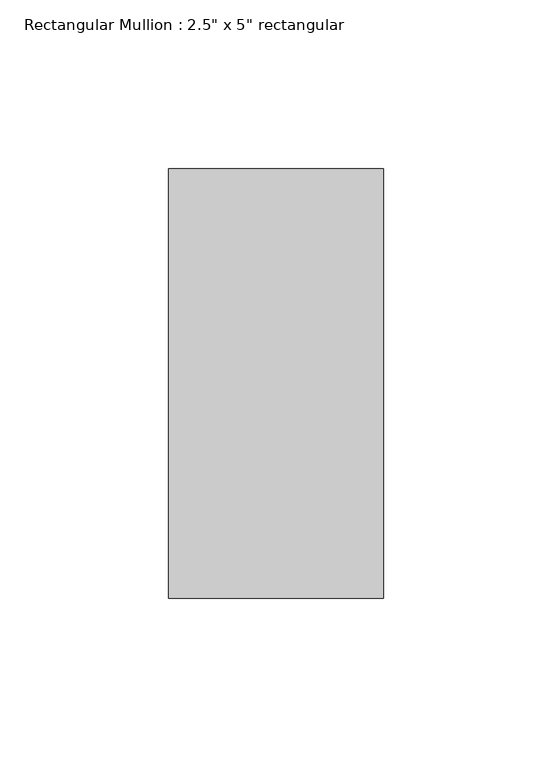
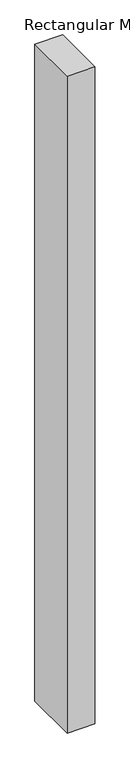
"""IFC4 building model written with IfcOpenShell, lengths in millimetres: member geometry."""

from ifc_helpers import new_model, si_unit, frame, origin, place, context, project, spatial, polyline, outline, extrude, source, transform, mapped, element, save


def member_af0bcaff(model_context):
    return source(origin(), model_context, "Body", "SweptSolid", [
        extrude(outline(polyline([(31.75, 63.5), (31.75, -63.5), (-31.75, -63.5), (-31.75, 63.5), (31.75, 63.5)])), frame((0.0, 0.0, -1582.9994987), z_axis=(0.0, 0.0, 1.0), x_axis=(1.0, 0.0, 0.0)), (0.0, 0.0, 1.0), 1582.9994987),
    ])


if __name__ == "__main__":
    model = new_model("IFC4")
    model_context = context("Model", 3, world=origin())
    ifc_project = project(units=[si_unit("LENGTHUNIT", "METRE", prefix="MILLI")], contexts=[model_context])
    site = spatial("IfcSite", under=ifc_project)
    building = spatial("IfcBuilding", under=site)
    placement = place(None, origin())
    member_shape = member_af0bcaff(model_context)
    element("IfcMember", 1, ObjectType="Rectangular Mullion : 2.5\" x 5\" rectangular", at=placement, inside=building, context=model_context, shape_type="MappedRepresentation", body=[
        mapped(member_shape, transform((0.0, 0.0, 0.0), x_axis=(1.0, 0.0, 0.0), y_axis=(0.0, 1.0, 0.0), z_axis=(0.0, 0.0, 1.0))),
    ])
    save(model, "model.ifc")

# Revit data of these elements
# Type "Rectangular Mullion : 2.5\" x 5\" rectangular"
#   built-in parameter 1007304 = 0.416667 (stored number, unit not read)
#   built-in parameter 1007301 = 0.104167 (stored number, unit not read)
#   built-in parameter 1007300 = 0.104167 (stored number, unit not read)
# Element 1 (IfcMember, "Rectangular Mullion : 2.5\" x 5\" rectangular")
#   Materials on its faces: "Aluminum"
# Materials
#   "Aluminum": class "Metal", colour RGB 247 247 247, transparency 0, Description = "Aluminum 6061", Cost = 0
